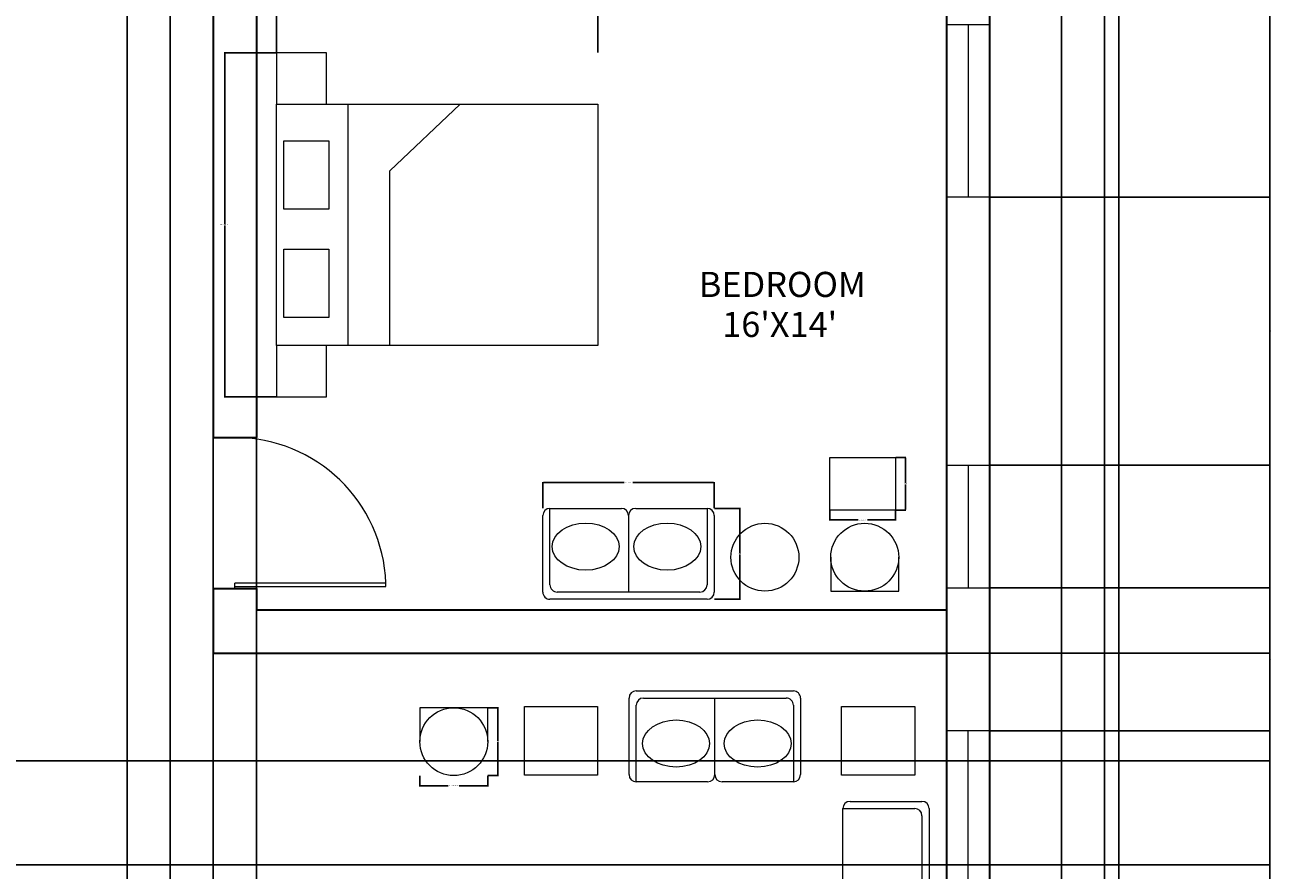
# Model space of a CAD drawing. Units: inches. Extents: x 2863 to 3499, y 1212 to 2136.
# Tile 6 of 7: x 3153 to 3499, y 1686 to 1921. Entities that reach past the tile are written whole.
import ezdxf

# ---------------------------------------------------------------- set-up
doc = ezdxf.new("R2010")
doc.units = ezdxf.units.IN
for name, color, linetype, lineweight in [('A-ANNO-DIMS', 2, 'Continuous', 18), ('A-AREA-IDEN', 7, 'Continuous', 18), ('A-DOOR', 221, 'Continuous', 18), ('A-FURN', 131, 'Continuous', 18), ('A-GLAZ', 191, 'Continuous', 18), ('A-WALL', 51, 'Continuous', 35), ('C-PROP', 51, 'Continuous', 25)]:
    doc.layers.add(name, color=color, linetype=linetype, lineweight=lineweight)
doc.styles.get("Standard").update_dxf_attribs({"font": 'arial.ttf'})
doc.dimstyles.get("Standard").update_dxf_attribs({"dimtxt": 0.18, "dimasz": 0.18, "dimexe": 0.18, "dimexo": 0.0625, "dimgap": 0.09, "dimtad": 0, "dimtih": 1, "dimtoh": 1, "dimdec": 4, "dimzin": 0, "dimdsep": 46, "dimtxsty": 'Standard', "dimcen": 0.09, "dimadec": 0, "dimazin": 0, "dimtfac": 1, "dimtdec": 4, "dimtofl": 0, "dimtmove": 0, "dimatfit": 3, "dimfxl": 1, "dimtolj": 1, "dimtzin": 0, "dimarcsym": 0})

# ---------------------------------------------------------------- blocks, each defined once
blk = doc.blocks.new('SOFA-TWO-SEAT')
for p, q in [((0, 45.71), (21.32, 45.71)), ((0, 25.85), (0, 45.71)), ((2, 47.71), (23.32, 47.71)), ((25.32, 45.71), (25.32, 2)), ((23.32, 43.71), (23.32, 4)), ((0, 2), (0, 21.85)), ((2, 23.85), (23.32, 23.85)), ((2, 23.85), (2, 23.85)), ((21.32, 2), (0, 2)), ((23.32, 0), (2, 0))]:
    blk.add_line(p, q)
for centre, start, end in [((2, 45.71), 90, 180), ((21.32, 43.71), 0, 90), ((23.32, 45.71), 0, 90), ((2, 25.85), 180, 270), ((2, 21.85), 90, 180), ((21.32, 4), 270, 0), ((2, 2), 180, 270), ((23.32, 2), 270, 0)]:
    blk.add_arc(centre, 2, start, end)
for centre in [(10.66, 34.63), (10.66, 11.93)]:
    blk.add_ellipse(centre, major_axis=(0, 9.3), ratio=0.704902)
blk = doc.blocks.new('BED-DOUBLE-WITH-NIGHTSTANDS')
for p, q in [((19.89, 14.28), (19.89, 81.52)), ((31.47, 62.91), (51.09, 81.52)), ((31.47, 14.28), (31.47, 62.91))]:
    blk.add_line(p, q)
for points in [[(0, 81.52), (13.89, 81.52), (13.89, 95.8), (0, 95.8)], [(0, 81.52), (89.37, 81.52), (89.37, 14.28), (0, 14.28)], [(2, 71.31), (14.52, 71.31), (14.52, 52.28), (2, 52.28)], [(2, 41.11), (14.52, 41.11), (14.52, 22.08), (2, 22.08)], [(0, 0), (13.89, 0), (13.89, 14.28), (0, 14.28)]]:
    blk.add_lwpolyline(points, close=True)
blk = doc.blocks.new('CHAIR-ROUND-BACK')
for p, q in [((18.9, 18.9), (0, 18.9)), ((0, 18.9), (0, 9.45)), ((18.9, 9.45), (18.9, 18.9))]:
    blk.add_line(p, q)
blk.add_circle((9.45, 9.45), 9.45)
blk = doc.blocks.new('TABLE-SIDE-ROUND')
blk.add_circle((9.45, 9.45), 9.45)
blk = doc.blocks.new('TABLE-SIDE-RECT')
blk.add_lwpolyline([(18.23, 14.69), (18.23, 0), (0, 0), (0, 14.69)], close=True)
blk = doc.blocks.new('TABLE-END-LOUNGE')
blk.add_lwpolyline([(0, 19.18), (20.36, 19.18), (20.36, 0), (0, 0)], close=True)
blk = doc.blocks.new('SOFA-THREE-SEAT')
for p, q in [((0, 2), (0, 22)), ((2, 24), (22, 24)), ((2, 4), (2, 24)), ((24, 22), (24, 2)), ((24, 22), (24, 22)), ((26, 24), (46, 24)), ((48, 22), (48, 2)), ((48, 22), (48, 22)), ((50, 24), (70, 24)), ((70, 24), (70, 4)), ((72, 22), (72, 2)), ((70, 0), (2, 0)), ((68, 2), (4, 2))]:
    blk.add_line(p, q)
for centre, start, end in [((2, 22), 90, 180), ((22, 22), 0, 90), ((26, 22), 90, 180), ((46, 22), 0, 90), ((50, 22), 90, 180), ((70, 22), 0, 90), ((4, 4), 180, 270), ((68, 4), 270, 0), ((2, 2), 180, 270), ((70, 2), 270, 0)]:
    blk.add_arc(centre, 2, start, end)
blk = doc.blocks.new('DOOR-SWING-42IN')
for p, q in [((42, 1.5), (0, 1.5)), ((0, 0.5), (0, 1.5)), ((0, 0), (0, 0.5)), ((0, 0.5), (42, 0.5)), ((42, 0.5), (42, 1.5))]:
    blk.add_line(p, q)
blk.add_arc((0.03, 0), 42, 2.0467, 90.0366)
blk = doc.blocks.new('WINDOW-48IN')
for p, q in [((12, 48), (0, 48)), ((6, 48), (6, 0)), ((12, 0), (0, 0))]:
    blk.add_line(p, q)
blk = doc.blocks.new('WINDOW-56IN')
for p, q in [((12, 56), (0, 56)), ((6, 0), (6, 56)), ((12, 0), (0, 0))]:
    blk.add_line(p, q)
blk = doc.blocks.new('*D19')
at = {"layer": 'A-ANNO-DIMS', "color": 0, "lineweight": -2, "transparency": 16777216}
for p, q in [((3296.61, 1786.52), (3296.61, 1793.79)), ((3296.79, 1793.61), (3319.24, 1793.61)), ((3344.14, 1793.61), (3321.69, 1793.61)), ((3344.32, 1786.52), (3344.32, 1793.79))]:
    blk.add_line(p, q, dxfattribs=at)
at = {"layer": 'A-ANNO-DIMS', "color": 0, "transparency": 16777216}
for points in [[(3296.79, 1793.64), (3296.79, 1793.58), (3296.61, 1793.61)], [(3344.14, 1793.64), (3344.14, 1793.58), (3344.32, 1793.61)]]:
    blk.add_solid(points, dxfattribs=at)
at = {"layer": 'Defpoints', "color": 0, "transparency": 16777216}
for p in [(3344.32, 1793.61), (3296.61, 1786.46), (3344.32, 1786.46)]:
    blk.add_point(p, dxfattribs=at)
at = {"layer": 'A-ANNO-DIMS', "color": 0, "transparency": 16777216, "insert": (3320.46, 1793.61), "char_height": 0.18, "attachment_point": 5}
blk.add_mtext('\\A1;LOVESEAT 48 TYP.', dxfattribs=at)
blk = doc.blocks.new('*D20')
at = {"layer": 'A-ANNO-DIMS', "color": 0, "lineweight": -2, "transparency": 16777216}
for p, q in [((3344.38, 1786.46), (3351.65, 1786.46)), ((3351.47, 1786.28), (3351.47, 1773.98)), ((3351.47, 1761.32), (3351.47, 1773.62)), ((3344.38, 1761.14), (3351.65, 1761.14))]:
    blk.add_line(p, q, dxfattribs=at)
at = {"layer": 'A-ANNO-DIMS', "color": 0, "transparency": 16777216}
for points in [[(3351.44, 1786.28), (3351.5, 1786.28), (3351.47, 1786.46)], [(3351.44, 1761.32), (3351.5, 1761.32), (3351.47, 1761.14)]]:
    blk.add_solid(points, dxfattribs=at)
at = {"layer": 'Defpoints', "color": 0, "transparency": 16777216}
for p in [(3344.32, 1786.46), (3344.32, 1761.14), (3351.47, 1761.14)]:
    blk.add_point(p, dxfattribs=at)
at = {"layer": 'A-ANNO-DIMS', "color": 0, "transparency": 16777216, "insert": (3351.47, 1773.8), "char_height": 0.18, "attachment_point": 5}
blk.add_mtext('\\A1;25 TYP.', dxfattribs=at)
blk = doc.blocks.new('*D21')
at = {"layer": 'A-ANNO-DIMS', "color": 0, "lineweight": -2, "transparency": 16777216}
for p, q in [((3262.39, 1711.98), (3262.39, 1709.03)), ((3281.29, 1711.98), (3281.29, 1709.03)), ((3262.57, 1709.21), (3270.32, 1709.21)), ((3281.11, 1709.21), (3273.35, 1709.21))]:
    blk.add_line(p, q, dxfattribs=at)
at = {"layer": 'A-ANNO-DIMS', "color": 0, "transparency": 16777216}
for points in [[(3262.57, 1709.24), (3262.57, 1709.18), (3262.39, 1709.21)], [(3281.11, 1709.24), (3281.11, 1709.18), (3281.29, 1709.21)]]:
    blk.add_solid(points, dxfattribs=at)
at = {"layer": 'Defpoints', "color": 0, "transparency": 16777216}
for p in [(3262.39, 1712.04), (3281.29, 1712.04), (3281.29, 1709.21)]:
    blk.add_point(p, dxfattribs=at)
at = {"layer": 'A-ANNO-DIMS', "color": 0, "transparency": 16777216, "insert": (3271.84, 1709.21), "char_height": 0.18, "attachment_point": 5}
blk.add_mtext('\\A1;LOUNGE CHAIR 19 TYP.', dxfattribs=at)
blk = doc.blocks.new('*D22')
at = {"layer": 'A-ANNO-DIMS', "color": 0, "lineweight": -2, "transparency": 16777216}
for p, q in [((3281.35, 1730.94), (3284.3, 1730.94)), ((3284.12, 1730.76), (3284.12, 1721.67)), ((3284.12, 1712.22), (3284.12, 1721.31)), ((3281.35, 1712.04), (3284.3, 1712.04))]:
    blk.add_line(p, q, dxfattribs=at)
at = {"layer": 'A-ANNO-DIMS', "color": 0, "transparency": 16777216}
for points in [[(3284.09, 1730.76), (3284.15, 1730.76), (3284.12, 1730.94)], [(3284.09, 1712.22), (3284.15, 1712.22), (3284.12, 1712.04)]]:
    blk.add_solid(points, dxfattribs=at)
at = {"layer": 'Defpoints', "color": 0, "transparency": 16777216}
for p in [(3281.29, 1730.94), (3284.12, 1730.94), (3281.29, 1712.04)]:
    blk.add_point(p, dxfattribs=at)
at = {"layer": 'A-ANNO-DIMS', "color": 0, "transparency": 16777216, "insert": (3284.12, 1721.49), "char_height": 0.18, "attachment_point": 5}
blk.add_mtext('\\A1;19 TYP.', dxfattribs=at)
blk = doc.blocks.new('*D27')
at = {"layer": 'A-ANNO-DIMS', "color": 0, "lineweight": -2, "transparency": 16777216}
for p, q in [((3376.51, 1785.91), (3376.51, 1783.06)), ((3394.74, 1785.91), (3394.74, 1783.06)), ((3376.69, 1783.24), (3384.34, 1783.24)), ((3394.56, 1783.24), (3386.92, 1783.24))]:
    blk.add_line(p, q, dxfattribs=at)
at = {"layer": 'A-ANNO-DIMS', "color": 0, "transparency": 16777216}
for points in [[(3376.69, 1783.27), (3376.69, 1783.21), (3376.51, 1783.24)], [(3394.56, 1783.27), (3394.56, 1783.21), (3394.74, 1783.24)]]:
    blk.add_solid(points, dxfattribs=at)
at = {"layer": 'Defpoints', "color": 0, "transparency": 16777216}
for p in [(3376.51, 1785.97), (3394.74, 1785.97), (3376.51, 1783.24)]:
    blk.add_point(p, dxfattribs=at)
at = {"layer": 'A-ANNO-DIMS', "color": 0, "transparency": 16777216, "insert": (3385.63, 1783.24), "char_height": 0.18, "attachment_point": 5}
blk.add_mtext('\\A1;SIDE TABLE 18 TYP.', dxfattribs=at)
blk = doc.blocks.new('*D28')
at = {"layer": 'A-ANNO-DIMS', "color": 0, "lineweight": -2, "transparency": 16777216}
for p, q in [((3394.8, 1800.66), (3397.66, 1800.66)), ((3397.48, 1800.48), (3397.48, 1793.5)), ((3397.48, 1786.15), (3397.48, 1793.13)), ((3394.8, 1785.97), (3397.66, 1785.97))]:
    blk.add_line(p, q, dxfattribs=at)
at = {"layer": 'A-ANNO-DIMS', "color": 0, "transparency": 16777216}
for points in [[(3397.45, 1800.48), (3397.51, 1800.48), (3397.48, 1800.66)], [(3397.45, 1786.15), (3397.51, 1786.15), (3397.48, 1785.97)]]:
    blk.add_solid(points, dxfattribs=at)
at = {"layer": 'Defpoints', "color": 0, "transparency": 16777216}
for p in [(3394.74, 1800.66), (3394.74, 1785.97), (3397.48, 1785.97)]:
    blk.add_point(p, dxfattribs=at)
at = {"layer": 'A-ANNO-DIMS', "color": 0, "transparency": 16777216, "insert": (3397.48, 1793.32), "char_height": 0.18, "attachment_point": 5}
blk.add_mtext('\\A1;15 TYP.', dxfattribs=at)
blk = doc.blocks.new('*D35')
at = {"layer": 'A-ANNO-DIMS', "color": 0, "lineweight": -2, "transparency": 16777216}
for p, q in [((3222.47, 1913.32), (3207.99, 1913.32)), ((3208.17, 1913.14), (3208.17, 1865.61)), ((3208.17, 1817.71), (3208.17, 1865.24)), ((3222.47, 1817.53), (3207.99, 1817.53))]:
    blk.add_line(p, q, dxfattribs=at)
at = {"layer": 'A-ANNO-DIMS', "color": 0, "transparency": 16777216}
for points in [[(3208.14, 1913.14), (3208.2, 1913.14), (3208.17, 1913.32)], [(3208.14, 1817.71), (3208.2, 1817.71), (3208.17, 1817.53)]]:
    blk.add_solid(points, dxfattribs=at)
at = {"layer": 'Defpoints', "color": 0, "transparency": 16777216}
for p in [(3208.17, 1913.32), (3222.54, 1913.32), (3222.54, 1817.53)]:
    blk.add_point(p, dxfattribs=at)
at = {"layer": 'A-ANNO-DIMS', "color": 0, "transparency": 16777216, "insert": (3208.17, 1865.43), "char_height": 0.18, "attachment_point": 5}
blk.add_mtext('\\A1;DOUBLE BED SET 96 TYP.', dxfattribs=at)
blk = doc.blocks.new('*D36')
at = {"layer": 'A-ANNO-DIMS', "color": 0, "lineweight": -2, "transparency": 16777216}
for p, q in [((3222.54, 1913.39), (3222.54, 1927.87)), ((3311.9, 1913.39), (3311.9, 1927.87)), ((3222.72, 1927.69), (3266.69, 1927.69)), ((3311.72, 1927.69), (3267.75, 1927.69))]:
    blk.add_line(p, q, dxfattribs=at)
at = {"layer": 'A-ANNO-DIMS', "color": 0, "transparency": 16777216}
for points in [[(3222.72, 1927.72), (3222.72, 1927.66), (3222.54, 1927.69)], [(3311.72, 1927.72), (3311.72, 1927.66), (3311.9, 1927.69)]]:
    blk.add_solid(points, dxfattribs=at)
at = {"layer": 'Defpoints', "color": 0, "transparency": 16777216}
for p in [(3311.9, 1927.69), (3222.54, 1913.32), (3311.9, 1913.32)]:
    blk.add_point(p, dxfattribs=at)
at = {"layer": 'A-ANNO-DIMS', "color": 0, "transparency": 16777216, "insert": (3267.22, 1927.69), "char_height": 0.18, "attachment_point": 5}
blk.add_mtext('\\A1;89 TYP.', dxfattribs=at)
blk = doc.blocks.new('*D57')
at = {"layer": 'A-ANNO-DIMS', "color": 0, "lineweight": -2, "transparency": 16777216}
for p, q in [((3456.98, 2094.17), (3499.12, 2094.17)), ((3498.94, 2093.99), (3498.94, 1734.35)), ((3498.94, 1374.35), (3498.94, 1733.98)), ((3452.98, 1374.17), (3499.12, 1374.17))]:
    blk.add_line(p, q, dxfattribs=at)
at = {"layer": 'A-ANNO-DIMS', "color": 0, "transparency": 16777216}
for points in [[(3498.91, 2093.99), (3498.97, 2093.99), (3498.94, 2094.17)], [(3498.91, 1374.35), (3498.97, 1374.35), (3498.94, 1374.17)]]:
    blk.add_solid(points, dxfattribs=at)
at = {"layer": 'Defpoints', "color": 0, "transparency": 16777216}
for p in [(3456.92, 2094.17), (3498.94, 2094.17), (3452.92, 1374.17)]:
    blk.add_point(p, dxfattribs=at)
at = {"layer": 'A-ANNO-DIMS', "color": 0, "transparency": 16777216, "insert": (3498.94, 1734.17), "char_height": 0.18, "attachment_point": 5}
blk.add_mtext('\\A1;720', dxfattribs=at)
blk = doc.blocks.new('*D60')
at = {"layer": 'A-ANNO-DIMS', "color": 0, "lineweight": -2, "transparency": 16777216}
for p, q in [((3408.98, 1746.17), (3499.12, 1746.17)), ((3498.94, 1745.99), (3498.94, 1647.85)), ((3498.94, 1549.35), (3498.94, 1647.48)), ((3408.98, 1549.17), (3499.12, 1549.17))]:
    blk.add_line(p, q, dxfattribs=at)
at = {"layer": 'A-ANNO-DIMS', "color": 0, "transparency": 16777216}
for points in [[(3498.91, 1745.99), (3498.97, 1745.99), (3498.94, 1746.17)], [(3498.91, 1549.35), (3498.97, 1549.35), (3498.94, 1549.17)]]:
    blk.add_solid(points, dxfattribs=at)
at = {"layer": 'Defpoints', "color": 0, "transparency": 16777216}
for p in [(3408.92, 1746.17), (3498.94, 1746.17), (3408.92, 1549.17)]:
    blk.add_point(p, dxfattribs=at)
at = {"layer": 'A-ANNO-DIMS', "color": 0, "transparency": 16777216, "insert": (3498.94, 1647.67), "char_height": 0.18, "attachment_point": 5}
blk.add_mtext('\\A1;197', dxfattribs=at)
blk = doc.blocks.new('*D61')
at = {"layer": 'A-ANNO-DIMS', "color": 0, "lineweight": -2, "transparency": 16777216}
for p, q in [((3408.98, 1926.17), (3499.12, 1926.17)), ((3498.94, 1925.99), (3498.94, 1836.35)), ((3498.94, 1746.35), (3498.94, 1835.98)), ((3408.98, 1746.17), (3499.12, 1746.17))]:
    blk.add_line(p, q, dxfattribs=at)
at = {"layer": 'A-ANNO-DIMS', "color": 0, "transparency": 16777216}
for points in [[(3498.91, 1925.99), (3498.97, 1925.99), (3498.94, 1926.17)], [(3498.91, 1746.35), (3498.97, 1746.35), (3498.94, 1746.17)]]:
    blk.add_solid(points, dxfattribs=at)
at = {"layer": 'Defpoints', "color": 0, "transparency": 16777216}
for p in [(3408.92, 1926.17), (3498.94, 1926.17), (3408.92, 1746.17)]:
    blk.add_point(p, dxfattribs=at)
at = {"layer": 'A-ANNO-DIMS', "color": 0, "transparency": 16777216, "insert": (3498.94, 1836.17), "char_height": 0.18, "attachment_point": 5}
blk.add_mtext('\\A1;180', dxfattribs=at)
blk = doc.blocks.new('*D72')
at = {"layer": 'A-ANNO-DIMS', "color": 0, "lineweight": -2, "transparency": 16777216}
for p, q in [((3133.92, 1549.23), (3133.92, 2136.37)), ((3134.1, 2136.19), (3169.22, 2136.19)), ((3204.74, 2136.19), (3169.62, 2136.19)), ((3204.92, 1561.23), (3204.92, 2136.37))]:
    blk.add_line(p, q, dxfattribs=at)
at = {"layer": 'A-ANNO-DIMS', "color": 0, "transparency": 16777216}
for points in [[(3134.1, 2136.22), (3134.1, 2136.16), (3133.92, 2136.19)], [(3204.74, 2136.22), (3204.74, 2136.16), (3204.92, 2136.19)]]:
    blk.add_solid(points, dxfattribs=at)
at = {"layer": 'Defpoints', "color": 0, "transparency": 16777216}
for p in [(3204.92, 2136.19), (3204.92, 1561.17), (3133.92, 1549.17)]:
    blk.add_point(p, dxfattribs=at)
at = {"layer": 'A-ANNO-DIMS', "color": 0, "transparency": 16777216, "insert": (3169.42, 2136.19), "char_height": 0.18, "attachment_point": 5}
blk.add_mtext('\\A1;71', dxfattribs=at)
blk = doc.blocks.new('*D96')
at = {"layer": 'A-ANNO-DIMS', "color": 0, "lineweight": -2, "transparency": 16777216}
for p, q in [((3420.98, 1764.31), (3499.12, 1764.31)), ((3498.94, 1764.13), (3498.94, 1744.58)), ((3498.94, 1724.67), (3498.94, 1744.22)), ((3420.98, 1724.49), (3499.12, 1724.49))]:
    blk.add_line(p, q, dxfattribs=at)
at = {"layer": 'A-ANNO-DIMS', "color": 0, "transparency": 16777216}
for points in [[(3498.91, 1764.13), (3498.97, 1764.13), (3498.94, 1764.31)], [(3498.91, 1724.67), (3498.97, 1724.67), (3498.94, 1724.49)]]:
    blk.add_solid(points, dxfattribs=at)
at = {"layer": 'Defpoints', "color": 0, "transparency": 16777216}
for p in [(3420.92, 1764.31), (3498.94, 1764.31), (3420.92, 1724.49)]:
    blk.add_point(p, dxfattribs=at)
at = {"layer": 'A-ANNO-DIMS', "color": 0, "transparency": 16777216, "insert": (3498.94, 1744.4), "char_height": 0.18, "attachment_point": 5}
blk.add_mtext('\\A1;39.82', dxfattribs=at)
blk = doc.blocks.new('*D97')
at = {"layer": 'A-ANNO-DIMS', "color": 0, "lineweight": -2, "transparency": 16777216}
for p, q in [((3420.98, 1798.51), (3499.12, 1798.51)), ((3498.94, 1798.33), (3498.94, 1781.59)), ((3498.94, 1764.49), (3498.94, 1781.23)), ((3420.98, 1764.31), (3499.12, 1764.31))]:
    blk.add_line(p, q, dxfattribs=at)
at = {"layer": 'A-ANNO-DIMS', "color": 0, "transparency": 16777216}
for points in [[(3498.91, 1798.33), (3498.97, 1798.33), (3498.94, 1798.51)], [(3498.91, 1764.49), (3498.97, 1764.49), (3498.94, 1764.31)]]:
    blk.add_solid(points, dxfattribs=at)
at = {"layer": 'Defpoints', "color": 0, "transparency": 16777216}
for p in [(3420.92, 1798.51), (3498.94, 1798.51), (3420.92, 1764.31)]:
    blk.add_point(p, dxfattribs=at)
at = {"layer": 'A-ANNO-DIMS', "color": 0, "transparency": 16777216, "insert": (3498.94, 1781.41), "char_height": 0.18, "attachment_point": 5}
blk.add_mtext('\\A1;34.2', dxfattribs=at)
blk = doc.blocks.new('*D98')
at = {"layer": 'A-ANNO-DIMS', "color": 0, "lineweight": -2, "transparency": 16777216}
for p, q in [((3420.98, 1873.08), (3499.12, 1873.08)), ((3498.94, 1872.9), (3498.94, 1835.98)), ((3498.94, 1798.69), (3498.94, 1835.62)), ((3420.98, 1798.51), (3499.12, 1798.51))]:
    blk.add_line(p, q, dxfattribs=at)
at = {"layer": 'A-ANNO-DIMS', "color": 0, "transparency": 16777216}
for points in [[(3498.91, 1872.9), (3498.97, 1872.9), (3498.94, 1873.08)], [(3498.91, 1798.69), (3498.97, 1798.69), (3498.94, 1798.51)]]:
    blk.add_solid(points, dxfattribs=at)
at = {"layer": 'Defpoints', "color": 0, "transparency": 16777216}
for p in [(3420.92, 1873.08), (3498.94, 1873.08), (3420.92, 1798.51)]:
    blk.add_point(p, dxfattribs=at)
at = {"layer": 'A-ANNO-DIMS', "color": 0, "transparency": 16777216, "insert": (3498.94, 1835.8), "char_height": 0.18, "attachment_point": 5}
blk.add_mtext('\\A1;74.57', dxfattribs=at)
blk = doc.blocks.new('*D107')
at = {"layer": 'A-ANNO-DIMS', "color": 0, "lineweight": -2, "transparency": 16777216}
for p, q in [((3216.92, 1270.23), (3216.92, 2136.37)), ((3217.1, 2136.19), (3328.63, 2136.19)), ((3440.74, 2136.19), (3329.21, 2136.19)), ((3440.92, 1270.23), (3440.92, 2136.37))]:
    blk.add_line(p, q, dxfattribs=at)
at = {"layer": 'A-ANNO-DIMS', "color": 0, "transparency": 16777216}
for points in [[(3217.1, 2136.22), (3217.1, 2136.16), (3216.92, 2136.19)], [(3440.74, 2136.22), (3440.74, 2136.16), (3440.92, 2136.19)]]:
    blk.add_solid(points, dxfattribs=at)
at = {"layer": 'Defpoints', "color": 0, "transparency": 16777216}
for p in [(3440.92, 2136.19), (3216.92, 1270.17), (3440.92, 1270.17)]:
    blk.add_point(p, dxfattribs=at)
at = {"layer": 'A-ANNO-DIMS', "color": 0, "transparency": 16777216, "insert": (3328.92, 2136.19), "char_height": 0.18, "attachment_point": 5}
blk.add_mtext('\\A1;224', dxfattribs=at)
blk = doc.blocks.new('*D110')
at = {"layer": 'A-ANNO-DIMS', "color": 0, "lineweight": -2, "transparency": 16777216}
for p, q in [((3180.92, 1374.23), (3180.92, 2136.37)), ((3181.1, 2136.19), (3186.71, 2136.19)), ((3192.74, 2136.19), (3187.13, 2136.19)), ((3192.92, 1374.23), (3192.92, 2136.37))]:
    blk.add_line(p, q, dxfattribs=at)
at = {"layer": 'A-ANNO-DIMS', "color": 0, "transparency": 16777216}
for points in [[(3181.1, 2136.22), (3181.1, 2136.16), (3180.92, 2136.19)], [(3192.74, 2136.22), (3192.74, 2136.16), (3192.92, 2136.19)]]:
    blk.add_solid(points, dxfattribs=at)
at = {"layer": 'Defpoints', "color": 0, "transparency": 16777216}
for p in [(3192.92, 2136.19), (3180.92, 1374.17), (3192.92, 1374.17)]:
    blk.add_point(p, dxfattribs=at)
at = {"layer": 'A-ANNO-DIMS', "color": 0, "transparency": 16777216, "insert": (3186.92, 2136.19), "char_height": 0.18, "attachment_point": 5}
blk.add_mtext('\\A1;12', dxfattribs=at)
blk = doc.blocks.new('*D113')
at = {"layer": 'A-ANNO-DIMS', "color": 0, "lineweight": -2, "transparency": 16777216}
for p, q in [((3085.72, 1716.17), (3499.12, 1716.17)), ((3498.94, 1715.99), (3498.94, 1701.85)), ((3498.94, 1687.35), (3498.94, 1701.48)), ((3085.72, 1687.17), (3499.12, 1687.17))]:
    blk.add_line(p, q, dxfattribs=at)
at = {"layer": 'A-ANNO-DIMS', "color": 0, "transparency": 16777216}
for points in [[(3498.91, 1715.99), (3498.97, 1715.99), (3498.94, 1716.17)], [(3498.91, 1687.35), (3498.97, 1687.35), (3498.94, 1687.17)]]:
    blk.add_solid(points, dxfattribs=at)
at = {"layer": 'Defpoints', "color": 0, "transparency": 16777216}
for p in [(3085.65, 1716.17), (3498.94, 1716.17), (3085.65, 1687.17)]:
    blk.add_point(p, dxfattribs=at)
at = {"layer": 'A-ANNO-DIMS', "color": 0, "transparency": 16777216, "insert": (3498.94, 1701.67), "char_height": 0.18, "attachment_point": 5}
blk.add_mtext('\\A1;29', dxfattribs=at)

msp = doc.modelspace()

# ---------------------------------------------------------------- linework, layer by layer
at = {"layer": 'A-GLAZ'}
for p, q in [((3408.9168, 1798.5136), (3420.9168, 1798.5136)), ((3414.9168, 1798.5136), (3414.9168, 1764.3109)), ((3408.9168, 1764.3109), (3420.9168, 1764.3109))]:
    msp.add_line(p, q, dxfattribs=at)
at = {"layer": 'A-WALL'}
for p, q in [((3204.9168, 1926.1651), (3204.9168, 1806.1651)), ((3216.9168, 1926.1651), (3216.9168, 1806.1651)), ((3408.9168, 1926.1651), (3408.9168, 1561.1651)), ((3204.9168, 1806.1651), (3216.9168, 1806.1651)), ((3204.9168, 1764.1651), (3216.9168, 1764.1651)), ((3204.9168, 1764.1651), (3204.9168, 1746.1651)), ((3216.9168, 1764.1651), (3216.9168, 1758.1651)), ((3216.9168, 1764.1651), (3216.9168, 1758.1651)), ((3216.9168, 1758.1651), (3408.9168, 1758.1651)), ((3204.9168, 1746.1651), (3408.9168, 1746.1651))]:
    msp.add_line(p, q, dxfattribs=at)
msp.add_lwpolyline([(2940.9168, 1453.1651), (2940.9168, 2094.1651), (3420.9168, 2094.1651), (3420.9168, 1374.1651), (3216.9168, 1374.1651)], dxfattribs=at)
at = {"layer": 'C-PROP'}
for p, q in [((3452.9168, 1258.1651), (3452.9168, 2094.1651)), ((3456.9168, 2094.1651), (3456.9168, 1254.1651))]:
    msp.add_line(p, q, dxfattribs=at)

# ---------------------------------------------------------------- block references
at = {"layer": 'A-DOOR'}
msp.add_blockref('DOOR-SWING-42IN', (3210.917, 1764.165), dxfattribs=at)
at = {"layer": 'A-FURN'}
for name, p in [('BED-DOUBLE-WITH-NIGHTSTANDS', (3222.5366, 1817.5275)), ('TABLE-SIDE-ROUND', (3348.9511, 1763.397)), ('CHAIR-ROUND-BACK', (3262.3903, 1712.0404)), ('TABLE-END-LOUNGE', (3291.5017, 1712.134)), ('TABLE-END-LOUNGE', (3379.75, 1712.134))]:
    msp.add_blockref(name, p, dxfattribs=at)
for name, p, rotation in [('TABLE-SIDE-RECT', (3394.7429, 1800.6592), 180), ('SOFA-TWO-SEAT', (3296.6078, 1786.4574), 269.9999999999976), ('CHAIR-ROUND-BACK', (3395.6319, 1782.2942), 180), ('SOFA-TWO-SEAT', (3368.3174, 1710.3053), 89.9999999999954), ('SOFA-THREE-SEAT', (3404.1005, 1632.8692), 89.99999999999898)]:
    msp.add_blockref(name, p, dxfattribs=dict(at, rotation=rotation))
at = {"layer": 'A-GLAZ'}
for name, p in [('WINDOW-48IN', (3408.917, 1873.0807)), ('WINDOW-56IN', (3408.917, 1668.4939))]:
    msp.add_blockref(name, p, dxfattribs=at)

# ---------------------------------------------------------------- texts
at = {"layer": 'A-AREA-IDEN'}
for tag, p in [('BEDROOM', (3340.0272, 1845.3155)), ("16'X14'", (3346.5287, 1834.1798))]:
    msp.add_attdef(tag, p, '', height=7, dxfattribs=at)

# ---------------------------------------------------------------- dimensions: what is measured, and where the dimension line sits
at = {"layer": 'A-ANNO-DIMS'}
for base, p1, p2, picture, middle in [((3204.9168, 2136.1851), (3133.9168, 1549.1651), (3204.9168, 1561.1651), '*D72', (3169.4168, 2136.1851)), ((3192.9168, 2136.1851), (3180.9168, 1374.1651), (3192.9168, 1374.1651), '*D110', (3186.9168, 2136.1851)), ((3440.9168, 2136.1851), (3216.9168, 1270.1651), (3440.9168, 1270.1651), '*D107', (3328.9168, 2136.1851))]:
    dim = msp.add_linear_dim(base=base, p1=p1, p2=p2, dimstyle='Standard', override={"dimdec": 0, "dimlfac": 1, "dimrnd": 0, "dimzin": 0, "dimdsep": 46, "dimlunit": 2}, dxfattribs=at)
    dim.commit()
    dim.dimension.update_dxf_attribs({"geometry": picture, "text_midpoint": middle})
for base, p1, p2, override, picture, middle in [((3498.9368, 2094.1651), (3452.9168, 1374.1651), (3456.9168, 2094.1651), {"dimdec": 0, "dimlfac": 1, "dimrnd": 0, "dimzin": 0, "dimdsep": 46, "dimlunit": 2}, '*D57', (3498.9368, 1734.1651)), ((3498.9368, 1926.1651), (3408.9168, 1746.1651), (3408.9168, 1926.1651), {"dimdec": 0, "dimlfac": 1, "dimrnd": 0, "dimzin": 0, "dimdsep": 46, "dimlunit": 2}, '*D61', (3498.9368, 1836.1651)), ((3498.9368, 1873.0807), (3420.9168, 1798.5136), (3420.9168, 1873.0807), {"dimdec": 2, "dimlfac": 1, "dimrnd": 0, "dimzin": 0, "dimdsep": 46, "dimlunit": 2}, '*D98', (3498.9368, 1835.7971)), ((3498.9368, 1798.5136), (3420.9168, 1764.3109), (3420.9168, 1798.5136), {"dimdec": 1, "dimlfac": 1, "dimrnd": 0, "dimzin": 0, "dimdsep": 46, "dimlunit": 2}, '*D97', (3498.9368, 1781.4122)), ((3498.9368, 1764.3109), (3420.9168, 1724.4934), (3420.9168, 1764.3109), {"dimdec": 2, "dimlfac": 1, "dimrnd": 0, "dimzin": 0, "dimdsep": 46, "dimlunit": 2}, '*D96', (3498.9368, 1744.4022)), ((3498.9368, 1746.1651), (3408.9168, 1549.1651), (3408.9168, 1746.1651), {"dimdec": 0, "dimlfac": 1, "dimrnd": 0, "dimzin": 0, "dimdsep": 46, "dimlunit": 2}, '*D60', (3498.9368, 1647.6651)), ((3498.9368, 1716.1651), (3085.6548, 1687.1651), (3085.6548, 1716.1651), {"dimdec": 0, "dimlfac": 1, "dimrnd": 0, "dimzin": 0, "dimdsep": 46, "dimlunit": 2}, '*D113', (3498.9368, 1701.6651))]:
    dim = msp.add_linear_dim(base=base, p1=p1, p2=p2, angle=90, dimstyle='Standard', override=override, dxfattribs=at)
    dim.commit()
    dim.dimension.update_dxf_attribs({"geometry": picture, "text_midpoint": middle})
for base, p1, p2, text, picture, middle in [((3311.9025, 1927.6929), (3222.5365, 1913.3235), (3311.9025, 1913.3235), '<> TYP.', '*D36', (3267.2195, 1927.6929)), ((3344.3161, 1793.614), (3296.6082, 1786.4578), (3344.3161, 1786.4578), 'LOVESEAT <> TYP.', '*D19', (3320.4621, 1793.614)), ((3281.2872, 1709.2059), (3262.3904, 1712.0404), (3281.2872, 1712.0404), 'LOUNGE CHAIR <> TYP.', '*D21', (3271.8388, 1709.2059))]:
    dim = msp.add_linear_dim(base=base, p1=p1, p2=p2, text=text, dimstyle='Standard', override={"dimdec": 0, "dimlfac": 1, "dimrnd": 0, "dimzin": 0, "dimdsep": 46, "dimlunit": 2}, dxfattribs=at)
    dim.commit()
    dim.dimension.update_dxf_attribs({"geometry": picture, "text_midpoint": middle})
for base, p1, p2, angle, text, picture, middle in [((3208.1671, 1913.3235), (3222.5365, 1817.5273), (3222.5365, 1913.3235), 90, 'DOUBLE BED SET <> TYP.', '*D35', (3208.1671, 1865.4254)), ((3397.4769, 1785.9737), (3394.7425, 1800.6591), (3394.7425, 1785.9737), 270, '<> TYP.', '*D28', (3397.4769, 1793.3164)), ((3351.4722, 1761.1413), (3344.3161, 1786.4578), (3344.3161, 1761.1413), 270, '<> TYP.', '*D20', (3351.4722, 1773.7996)), ((3376.5126, 1783.2392), (3394.7425, 1785.9737), (3376.5126, 1785.9737), 180, 'SIDE TABLE <> TYP.', '*D27', (3385.6275, 1783.2392)), ((3284.1218, 1730.9372), (3281.2872, 1712.0404), (3281.2872, 1730.9372), 90, '<> TYP.', '*D22', (3284.1218, 1721.4888))]:
    dim = msp.add_linear_dim(base=base, p1=p1, p2=p2, angle=angle, text=text, dimstyle='Standard', override={"dimdec": 0, "dimlfac": 1, "dimrnd": 0, "dimzin": 0, "dimdsep": 46, "dimlunit": 2}, dxfattribs=at)
    dim.commit()
    dim.dimension.update_dxf_attribs({"geometry": picture, "text_midpoint": middle})

doc.saveas('drawing.dxf')
